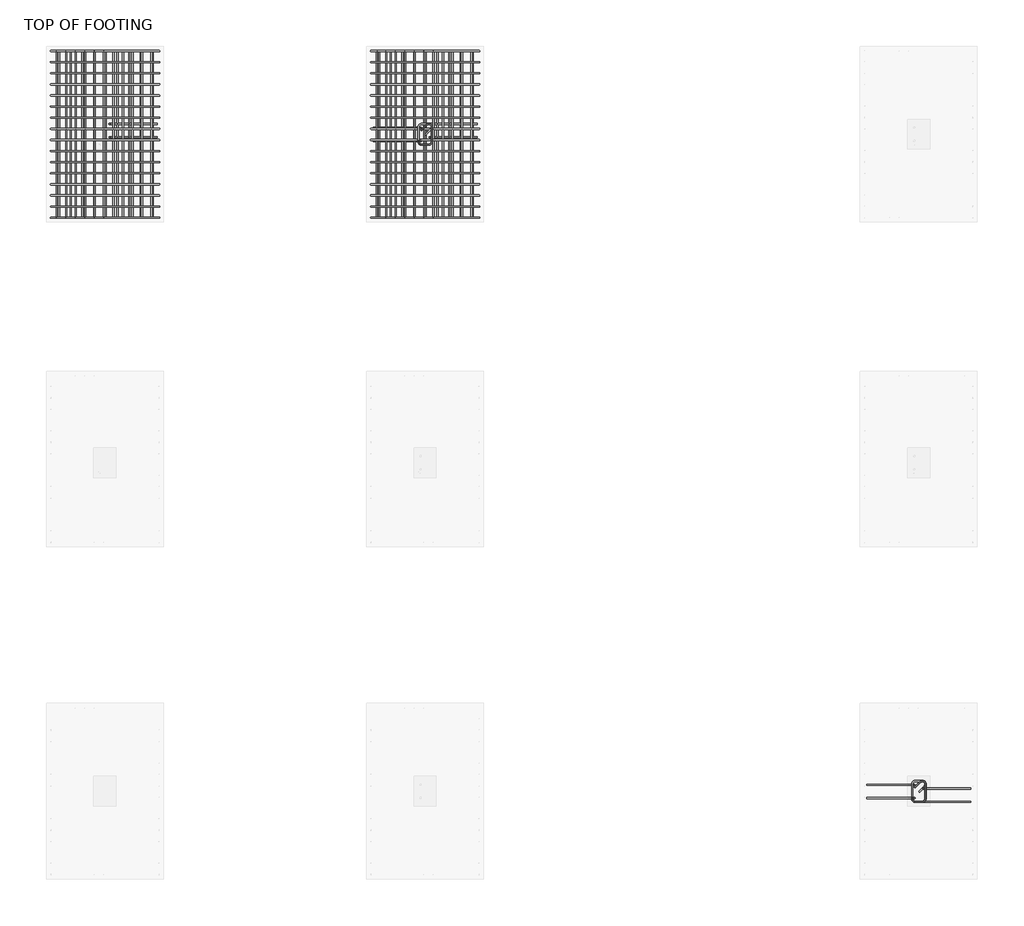
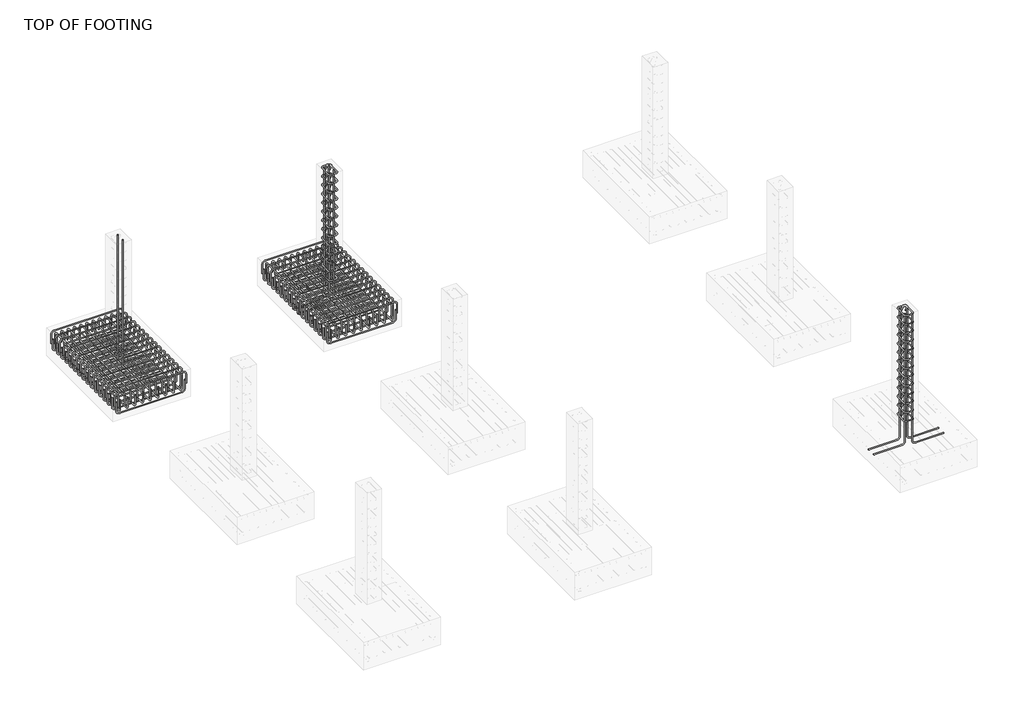
# One storey, part 4 of 8: 15 reinforcing bars.
"""IFC4 building model written with IfcOpenShell, lengths in millimetres."""

from ifc_helpers import new_model, si_unit, point, frame, origin, place, context, project, spatial, polyline, circle_curve, trimmed, segment, composite_curve, source, transform, mapped, element, save
from ifc_brep_helpers import swept_disk

model = new_model("IFC4")

# Units and contexts
model_context = context("Model", 3, world=origin())
ifc_project = project(units=[si_unit("LENGTHUNIT", "METRE", prefix="MILLI")], contexts=[model_context])

# Site, building, storey
site = spatial("IfcSite", under=ifc_project)
building = spatial("IfcBuilding", under=site)
storey = spatial("IfcBuildingStorey", under=building, Name="TOP OF FOOTING", Elevation=-1828.8)

# Reinforcing bars
placement = place(None, origin())
reinforcing_bar_shape = source(origin(), model_context, "Body", "SolidModel", [
    swept_disk(composite_curve([segment(polyline([(-4695.380398, 8895.4265586, -2177.1384798), (-5136.5372203, 8895.4265586, -2177.1384798)]), True, "CONTINUOUS"), segment(trimmed(circle_curve(frame((-5136.5372203, 8895.4265586, -2130.7884798), z_axis=(0.0, 1.0, 0.0), x_axis=(0.0, 0.0, -46.34999999999991)), 46.35), [point((-5136.5372203, 8895.4265586, -2177.1384798))], [point((-5182.8872203, 8895.4265586, -2130.7884798))], True, "CARTESIAN"), True, "CONTINUOUS"), segment(polyline([(-5182.8872203, 8895.4265586, -2130.7884798), (-5182.8872203, 8895.4265586, -40.0)]), True, "CONTINUOUS")], self_intersect=False), 6.35),
])
element("IfcReinforcingBar", 1, at=placement, inside=storey, context=model_context, shape_type="MappedRepresentation", body=[
    mapped(reinforcing_bar_shape, transform((0.0, 0.0, 0.0), x_axis=(1.0, 0.0, 0.0), y_axis=(0.0, 1.0, 0.0), z_axis=(0.0, 0.0, 1.0))),
    mapped(reinforcing_bar_shape, transform((0.0, 135.9, 0.0), x_axis=(1.0, 0.0, 0.0), y_axis=(0.0, 1.0, 0.0), z_axis=(0.0, 0.0, 1.0))),
])
reinforcing_bar_2_shape = source(origin(), model_context, "Body", "SolidModel", [
    swept_disk(composite_curve([segment(polyline([(-1993.1182423, 8966.4007933, -46.35), (-1937.3746793, 9022.1443562, -46.35)]), True, "CONTINUOUS"), segment(trimmed(circle_curve(frame((-1915.2068817, 8999.9765586, -46.35), z_axis=(0.0, 0.0, -1.0), x_axis=(-22.167797600000085, 22.167797600000995, 0.0)), 31.35), [point((-1937.3746793, 9022.1443562, -46.35))], [point((-1883.8568817, 8999.9765586, -46.35))], True, "CARTESIAN"), True, "CONTINUOUS"), segment(polyline([(-1883.8568817, 8999.9765586, -46.35), (-1883.8568817, 8850.5765586, -46.35)]), True, "CONTINUOUS"), segment(trimmed(circle_curve(frame((-1915.2068817, 8850.5765586, -46.35), z_axis=(0.0, 0.0, -1.0), x_axis=(31.34999999999991, 0.0, 0.0)), 31.35), [point((-1883.8568817, 8850.5765586, -46.35))], [point((-1915.2068817, 8819.2265586, -46.35))], True, "CARTESIAN"), True, "CONTINUOUS"), segment(polyline([(-1915.2068817, 8819.2265586, -46.35), (-1988.4068817, 8819.2265586, -46.35)]), True, "CONTINUOUS"), segment(trimmed(circle_curve(frame((-1988.4068817, 8850.5205096, -44.4761991), z_axis=(0.0, 0.05977036468717588, -0.9982121535551258), x_axis=(0.0, -31.29395100000147, -1.873800899999999)), 31.35), [point((-1988.4068817, 8819.2265586, -46.35))], [point((-2019.7568817, 8850.5205096, -44.4761991))], True, "CARTESIAN"), True, "CONTINUOUS"), segment(polyline([(-2019.7568817, 8850.5205096, -44.4761991), (-2019.7568817, 9000.0326076, -35.5238009)]), True, "CONTINUOUS"), segment(trimmed(circle_curve(frame((-1988.4068817, 9000.0326076, -35.5238009), z_axis=(0.0, 0.05977036468717588, -0.9982121535551258), x_axis=(-31.34999999999991, 0.0, 0.0)), 31.35), [point((-2019.7568817, 9000.0326076, -35.5238009))], [point((-1988.4068817, 9031.3265586, -33.65))], True, "CARTESIAN"), True, "CONTINUOUS"), segment(polyline([(-1988.4068817, 9031.3265586, -33.65), (-1915.2068817, 9031.3265586, -33.65)]), True, "CONTINUOUS"), segment(trimmed(circle_curve(frame((-1915.2068817, 8999.9765586, -33.65), z_axis=(0.0, 0.0, -1.0), x_axis=(0.0, 31.350000000000364, 0.0)), 31.35), [point((-1915.2068817, 9031.3265586, -33.65))], [point((-1893.0390841, 8977.808761, -33.65))], True, "CARTESIAN"), True, "CONTINUOUS"), segment(polyline([(-1893.0390841, 8977.808761, -33.65), (-1948.7826471, 8922.0651981, -33.65)]), True, "CONTINUOUS")], self_intersect=False), 6.35),
])
element("IfcReinforcingBar", 2, at=placement, inside=storey, context=model_context, shape_type="MappedRepresentation", body=[
    mapped(reinforcing_bar_2_shape, transform((0.0, 0.0, 0.0), x_axis=(1.0, 0.0, 0.0), y_axis=(0.0, 1.0, 0.0), z_axis=(0.0, 0.0, 1.0))),
    mapped(reinforcing_bar_2_shape, transform((0.0, 0.0, -144.675), x_axis=(1.0, 0.0, 0.0), y_axis=(0.0, 1.0, 0.0), z_axis=(0.0, 0.0, 1.0))),
    mapped(reinforcing_bar_2_shape, transform((0.0, 0.0, -289.35), x_axis=(1.0, 0.0, 0.0), y_axis=(0.0, 1.0, 0.0), z_axis=(0.0, 0.0, 1.0))),
    mapped(reinforcing_bar_2_shape, transform((0.0, 0.0, -434.025), x_axis=(1.0, 0.0, 0.0), y_axis=(0.0, 1.0, 0.0), z_axis=(0.0, 0.0, 1.0))),
    mapped(reinforcing_bar_2_shape, transform((0.0, 0.0, -578.7), x_axis=(1.0, 0.0, 0.0), y_axis=(0.0, 1.0, 0.0), z_axis=(0.0, 0.0, 1.0))),
    mapped(reinforcing_bar_2_shape, transform((0.0, 0.0, -723.375), x_axis=(1.0, 0.0, 0.0), y_axis=(0.0, 1.0, 0.0), z_axis=(0.0, 0.0, 1.0))),
    mapped(reinforcing_bar_2_shape, transform((0.0, 0.0, -868.05), x_axis=(1.0, 0.0, 0.0), y_axis=(0.0, 1.0, 0.0), z_axis=(0.0, 0.0, 1.0))),
    mapped(reinforcing_bar_2_shape, transform((0.0, 0.0, -1012.725), x_axis=(1.0, 0.0, 0.0), y_axis=(0.0, 1.0, 0.0), z_axis=(0.0, 0.0, 1.0))),
    mapped(reinforcing_bar_2_shape, transform((0.0, 0.0, -1157.4), x_axis=(1.0, 0.0, 0.0), y_axis=(0.0, 1.0, 0.0), z_axis=(0.0, 0.0, 1.0))),
    mapped(reinforcing_bar_2_shape, transform((0.0, 0.0, -1302.075), x_axis=(1.0, 0.0, 0.0), y_axis=(0.0, 1.0, 0.0), z_axis=(0.0, 0.0, 1.0))),
    mapped(reinforcing_bar_2_shape, transform((0.0, 0.0, -1446.75), x_axis=(1.0, 0.0, 0.0), y_axis=(0.0, 1.0, 0.0), z_axis=(0.0, 0.0, 1.0))),
    mapped(reinforcing_bar_2_shape, transform((0.0, 0.0, -1591.425), x_axis=(1.0, 0.0, 0.0), y_axis=(0.0, 1.0, 0.0), z_axis=(0.0, 0.0, 1.0))),
    mapped(reinforcing_bar_2_shape, transform((0.0, 0.0, -1736.1), x_axis=(1.0, 0.0, 0.0), y_axis=(0.0, 1.0, 0.0), z_axis=(0.0, 0.0, 1.0))),
])
reinforcing_bar_3_shape = source(origin(), model_context, "Body", "SolidModel", [
    swept_disk(composite_curve([segment(polyline([(-1418.780398, 8895.4265586, -2177.1384798), (-1859.9372203, 8895.4265586, -2177.1384798)]), True, "CONTINUOUS"), segment(trimmed(circle_curve(frame((-1859.9372203, 8895.4265586, -2130.7884798), z_axis=(0.0, 1.0, 0.0), x_axis=(0.0, 0.0, -46.34999999999991)), 46.35), [point((-1859.9372203, 8895.4265586, -2177.1384798))], [point((-1906.2872203, 8895.4265586, -2130.7884798))], True, "CARTESIAN"), True, "CONTINUOUS"), segment(polyline([(-1906.2872203, 8895.4265586, -2130.7884798), (-1906.2872203, 8895.4265586, -40.0)]), True, "CONTINUOUS")], self_intersect=False), 6.35),
])
element("IfcReinforcingBar", 3, at=placement, inside=storey, context=model_context, shape_type="MappedRepresentation", body=[
    mapped(reinforcing_bar_3_shape, transform((0.0, 0.0, 0.0), x_axis=(1.0, 0.0, 0.0), y_axis=(0.0, 1.0, 0.0), z_axis=(0.0, 0.0, 1.0))),
    mapped(reinforcing_bar_3_shape, transform((0.0, 135.9, 0.0), x_axis=(1.0, 0.0, 0.0), y_axis=(0.0, 1.0, 0.0), z_axis=(0.0, 0.0, 1.0))),
])
reinforcing_bar_4_shape = source(origin(), model_context, "Body", "SolidModel", [
    swept_disk(composite_curve([segment(polyline([(-2484.8333654, 8857.3265586, -2177.1384798), (-2043.6765432, 8857.3265586, -2177.1384798)]), True, "CONTINUOUS"), segment(trimmed(circle_curve(frame((-2043.6765432, 8857.3265586, -2130.7884798), z_axis=(0.0, -1.0, 0.0), x_axis=(0.0, 0.0, -46.34999999999991)), 46.35), [point((-2043.6765432, 8857.3265586, -2177.1384798))], [point((-1997.3265432, 8857.3265586, -2130.7884798))], True, "CARTESIAN"), True, "CONTINUOUS"), segment(polyline([(-1997.3265432, 8857.3265586, -2130.7884798), (-1997.3265432, 8857.3265586, -40.0)]), True, "CONTINUOUS")], self_intersect=False), 6.35),
])
element("IfcReinforcingBar", 4, at=placement, inside=storey, context=model_context, shape_type="MappedRepresentation", body=[
    mapped(reinforcing_bar_4_shape, transform((0.0, 0.0, 0.0), x_axis=(1.0, 0.0, 0.0), y_axis=(0.0, 1.0, 0.0), z_axis=(0.0, 0.0, 1.0))),
    mapped(reinforcing_bar_4_shape, transform((0.0, 135.9, 0.0), x_axis=(1.0, 0.0, 0.0), y_axis=(0.0, 1.0, 0.0), z_axis=(0.0, 0.0, 1.0))),
])
reinforcing_bar_5_shape = source(origin(), model_context, "Body", "SolidModel", [
    swept_disk(composite_curve([segment(polyline([(3061.4817577, 2235.4007933, -46.35), (3117.2253207, 2291.1443562, -46.35)]), True, "CONTINUOUS"), segment(trimmed(circle_curve(frame((3139.3931183, 2268.9765586, -46.35), z_axis=(0.0, 0.0, -1.0), x_axis=(-22.167797600000085, 22.167797600000085, 0.0)), 31.35), [point((3117.2253207, 2291.1443562, -46.35))], [point((3170.7431183, 2268.9765586, -46.35))], True, "CARTESIAN"), True, "CONTINUOUS"), segment(polyline([(3170.7431183, 2268.9765586, -46.35), (3170.7431183, 2119.5765586, -46.35)]), True, "CONTINUOUS"), segment(trimmed(circle_curve(frame((3139.3931183, 2119.5765586, -46.35), z_axis=(0.0, 0.0, -1.0), x_axis=(31.34999999999991, 0.0, 0.0)), 31.35), [point((3170.7431183, 2119.5765586, -46.35))], [point((3139.3931183, 2088.2265586, -46.35))], True, "CARTESIAN"), True, "CONTINUOUS"), segment(polyline([(3139.3931183, 2088.2265586, -46.35), (3066.1931183, 2088.2265586, -46.35)]), True, "CONTINUOUS"), segment(trimmed(circle_curve(frame((3066.1931183, 2119.5205096, -44.4761991), z_axis=(0.0, 0.05977036468717588, -0.9982121535551258), x_axis=(0.0, -31.293951000000106, -1.873800899999999)), 31.35), [point((3066.1931183, 2088.2265586, -46.35))], [point((3034.8431183, 2119.5205096, -44.4761991))], True, "CARTESIAN"), True, "CONTINUOUS"), segment(polyline([(3034.8431183, 2119.5205096, -44.4761991), (3034.8431183, 2269.0326076, -35.5238009)]), True, "CONTINUOUS"), segment(trimmed(circle_curve(frame((3066.1931183, 2269.0326076, -35.5238009), z_axis=(0.0, 0.05977036468717588, -0.9982121535551258), x_axis=(-31.350000000000364, 0.0, 0.0)), 31.35), [point((3034.8431183, 2269.0326076, -35.5238009))], [point((3066.1931183, 2300.3265586, -33.65))], True, "CARTESIAN"), True, "CONTINUOUS"), segment(polyline([(3066.1931183, 2300.3265586, -33.65), (3139.3931183, 2300.3265586, -33.65)]), True, "CONTINUOUS"), segment(trimmed(circle_curve(frame((3139.3931183, 2268.9765586, -33.65), z_axis=(0.0, 0.0, -1.0), x_axis=(0.0, 31.350000000000364, 0.0)), 31.35), [point((3139.3931183, 2300.3265586, -33.65))], [point((3161.5609159, 2246.808761, -33.65))], True, "CARTESIAN"), True, "CONTINUOUS"), segment(polyline([(3161.5609159, 2246.808761, -33.65), (3105.8173529, 2191.0651981, -33.65)]), True, "CONTINUOUS")], self_intersect=False), 6.35),
])
element("IfcReinforcingBar", 5, at=placement, inside=storey, context=model_context, shape_type="MappedRepresentation", body=[
    mapped(reinforcing_bar_5_shape, transform((0.0, 0.0, 0.0), x_axis=(1.0, 0.0, 0.0), y_axis=(0.0, 1.0, 0.0), z_axis=(0.0, 0.0, 1.0))),
    mapped(reinforcing_bar_5_shape, transform((0.0, 0.0, -144.675), x_axis=(1.0, 0.0, 0.0), y_axis=(0.0, 1.0, 0.0), z_axis=(0.0, 0.0, 1.0))),
    mapped(reinforcing_bar_5_shape, transform((0.0, 0.0, -289.35), x_axis=(1.0, 0.0, 0.0), y_axis=(0.0, 1.0, 0.0), z_axis=(0.0, 0.0, 1.0))),
    mapped(reinforcing_bar_5_shape, transform((0.0, 0.0, -434.025), x_axis=(1.0, 0.0, 0.0), y_axis=(0.0, 1.0, 0.0), z_axis=(0.0, 0.0, 1.0))),
    mapped(reinforcing_bar_5_shape, transform((0.0, 0.0, -578.7), x_axis=(1.0, 0.0, 0.0), y_axis=(0.0, 1.0, 0.0), z_axis=(0.0, 0.0, 1.0))),
    mapped(reinforcing_bar_5_shape, transform((0.0, 0.0, -723.375), x_axis=(1.0, 0.0, 0.0), y_axis=(0.0, 1.0, 0.0), z_axis=(0.0, 0.0, 1.0))),
    mapped(reinforcing_bar_5_shape, transform((0.0, 0.0, -868.05), x_axis=(1.0, 0.0, 0.0), y_axis=(0.0, 1.0, 0.0), z_axis=(0.0, 0.0, 1.0))),
    mapped(reinforcing_bar_5_shape, transform((0.0, 0.0, -1012.725), x_axis=(1.0, 0.0, 0.0), y_axis=(0.0, 1.0, 0.0), z_axis=(0.0, 0.0, 1.0))),
    mapped(reinforcing_bar_5_shape, transform((0.0, 0.0, -1157.4), x_axis=(1.0, 0.0, 0.0), y_axis=(0.0, 1.0, 0.0), z_axis=(0.0, 0.0, 1.0))),
    mapped(reinforcing_bar_5_shape, transform((0.0, 0.0, -1302.075), x_axis=(1.0, 0.0, 0.0), y_axis=(0.0, 1.0, 0.0), z_axis=(0.0, 0.0, 1.0))),
    mapped(reinforcing_bar_5_shape, transform((0.0, 0.0, -1446.75), x_axis=(1.0, 0.0, 0.0), y_axis=(0.0, 1.0, 0.0), z_axis=(0.0, 0.0, 1.0))),
    mapped(reinforcing_bar_5_shape, transform((0.0, 0.0, -1591.425), x_axis=(1.0, 0.0, 0.0), y_axis=(0.0, 1.0, 0.0), z_axis=(0.0, 0.0, 1.0))),
    mapped(reinforcing_bar_5_shape, transform((0.0, 0.0, -1736.1), x_axis=(1.0, 0.0, 0.0), y_axis=(0.0, 1.0, 0.0), z_axis=(0.0, 0.0, 1.0))),
])
reinforcing_bar_6_shape = source(origin(), model_context, "Body", "SolidModel", [
    swept_disk(composite_curve([segment(polyline([(3635.819602, 2088.2265586, -2177.1384798), (3194.6627797, 2088.2265586, -2177.1384798)]), True, "CONTINUOUS"), segment(trimmed(circle_curve(frame((3194.6627797, 2088.2265586, -2130.7884798), z_axis=(0.0, 1.0, 0.0), x_axis=(0.0, 0.0, -46.34999999999991)), 46.35), [point((3194.6627797, 2088.2265586, -2177.1384798))], [point((3148.3127797, 2088.2265586, -2130.7884798))], True, "CARTESIAN"), True, "CONTINUOUS"), segment(polyline([(3148.3127797, 2088.2265586, -2130.7884798), (3148.3127797, 2088.2265586, -40.0)]), True, "CONTINUOUS")], self_intersect=False), 6.35),
])
element("IfcReinforcingBar", 6, at=placement, inside=storey, context=model_context, shape_type="MappedRepresentation", body=[
    mapped(reinforcing_bar_6_shape, transform((0.0, 0.0, 0.0), x_axis=(1.0, 0.0, 0.0), y_axis=(0.0, 1.0, 0.0), z_axis=(0.0, 0.0, 1.0))),
    mapped(reinforcing_bar_6_shape, transform((0.0, 135.9, 0.0), x_axis=(1.0, 0.0, 0.0), y_axis=(0.0, 1.0, 0.0), z_axis=(0.0, 0.0, 1.0))),
])
reinforcing_bar_7_shape = source(origin(), model_context, "Body", "SolidModel", [
    swept_disk(composite_curve([segment(polyline([(2569.7666346, 2126.3265586, -2177.1384798), (3010.9234568, 2126.3265586, -2177.1384798)]), True, "CONTINUOUS"), segment(trimmed(circle_curve(frame((3010.9234568, 2126.3265586, -2130.7884798), z_axis=(0.0, -1.0, 0.0), x_axis=(0.0, 0.0, -46.34999999999991)), 46.35), [point((3010.9234568, 2126.3265586, -2177.1384798))], [point((3057.2734568, 2126.3265586, -2130.7884798))], True, "CARTESIAN"), True, "CONTINUOUS"), segment(polyline([(3057.2734568, 2126.3265586, -2130.7884798), (3057.2734568, 2126.3265586, -40.0)]), True, "CONTINUOUS")], self_intersect=False), 6.35),
])
element("IfcReinforcingBar", 7, at=placement, inside=storey, context=model_context, shape_type="MappedRepresentation", body=[
    mapped(reinforcing_bar_7_shape, transform((0.0, 0.0, 0.0), x_axis=(1.0, 0.0, 0.0), y_axis=(0.0, 1.0, 0.0), z_axis=(0.0, 0.0, 1.0))),
    mapped(reinforcing_bar_7_shape, transform((0.0, 135.9, 0.0), x_axis=(1.0, 0.0, 0.0), y_axis=(0.0, 1.0, 0.0), z_axis=(0.0, 0.0, 1.0))),
])
reinforcing_bar_8_shape = source(origin(), model_context, "Body", "SolidModel", [
    swept_disk(composite_curve([segment(polyline([(-4694.1573229, 9778.9265586, -2008.2544267), (-4694.1573229, 9778.9265586, -2155.5544267)]), True, "CONTINUOUS"), segment(trimmed(circle_curve(frame((-4740.5073229, 9778.9265586, -2155.5544267), z_axis=(0.0, 1.0, 0.0), x_axis=(46.350000000000364, 0.0, 0.0)), 46.35), [point((-4694.1573229, 9778.9265586, -2155.5544267))], [point((-4740.5073229, 9778.9265586, -2201.9044267))], True, "CARTESIAN"), True, "CONTINUOUS"), segment(polyline([(-4740.5073229, 9778.9265586, -2201.9044267), (-5711.5233592, 9778.9265586, -2201.9044267)]), True, "CONTINUOUS"), segment(trimmed(circle_curve(frame((-5711.5233592, 9778.9265586, -2155.5544267), z_axis=(0.0, 1.0, 0.0), x_axis=(0.0, 0.0, -46.34999999999991)), 46.35), [point((-5711.5233592, 9778.9265586, -2201.9044267))], [point((-5757.8733592, 9778.9265586, -2155.5544267))], True, "CARTESIAN"), True, "CONTINUOUS"), segment(polyline([(-5757.8733592, 9778.9265586, -2155.5544267), (-5757.8733592, 9778.9265586, -2008.2544267)]), True, "CONTINUOUS")], self_intersect=False), 6.35),
])
element("IfcReinforcingBar", 8, at=placement, inside=storey, context=model_context, shape_type="MappedRepresentation", body=[
    mapped(reinforcing_bar_8_shape, transform((0.0, 0.0, 0.0), x_axis=(1.0, 0.0, 0.0), y_axis=(0.0, 1.0, 0.0), z_axis=(0.0, 0.0, 1.0))),
    mapped(reinforcing_bar_8_shape, transform((0.0, -113.82, 0.0), x_axis=(1.0, 0.0, 0.0), y_axis=(0.0, 1.0, 0.0), z_axis=(0.0, 0.0, 1.0))),
    mapped(reinforcing_bar_8_shape, transform((0.0, -227.64, 0.0), x_axis=(1.0, 0.0, 0.0), y_axis=(0.0, 1.0, 0.0), z_axis=(0.0, 0.0, 1.0))),
    mapped(reinforcing_bar_8_shape, transform((0.0, -341.46, 0.0), x_axis=(1.0, 0.0, 0.0), y_axis=(0.0, 1.0, 0.0), z_axis=(0.0, 0.0, 1.0))),
    mapped(reinforcing_bar_8_shape, transform((0.0, -455.28, 0.0), x_axis=(1.0, 0.0, 0.0), y_axis=(0.0, 1.0, 0.0), z_axis=(0.0, 0.0, 1.0))),
    mapped(reinforcing_bar_8_shape, transform((0.0, -569.1, 0.0), x_axis=(1.0, 0.0, 0.0), y_axis=(0.0, 1.0, 0.0), z_axis=(0.0, 0.0, 1.0))),
    mapped(reinforcing_bar_8_shape, transform((0.0, -682.92, 0.0), x_axis=(1.0, 0.0, 0.0), y_axis=(0.0, 1.0, 0.0), z_axis=(0.0, 0.0, 1.0))),
    mapped(reinforcing_bar_8_shape, transform((0.0, -796.74, 0.0), x_axis=(1.0, 0.0, 0.0), y_axis=(0.0, 1.0, 0.0), z_axis=(0.0, 0.0, 1.0))),
    mapped(reinforcing_bar_8_shape, transform((0.0, -910.56, 0.0), x_axis=(1.0, 0.0, 0.0), y_axis=(0.0, 1.0, 0.0), z_axis=(0.0, 0.0, 1.0))),
    mapped(reinforcing_bar_8_shape, transform((0.0, -1024.38, 0.0), x_axis=(1.0, 0.0, 0.0), y_axis=(0.0, 1.0, 0.0), z_axis=(0.0, 0.0, 1.0))),
    mapped(reinforcing_bar_8_shape, transform((0.0, -1138.2, 0.0), x_axis=(1.0, 0.0, 0.0), y_axis=(0.0, 1.0, 0.0), z_axis=(0.0, 0.0, 1.0))),
    mapped(reinforcing_bar_8_shape, transform((0.0, -1252.02, 0.0), x_axis=(1.0, 0.0, 0.0), y_axis=(0.0, 1.0, 0.0), z_axis=(0.0, 0.0, 1.0))),
    mapped(reinforcing_bar_8_shape, transform((0.0, -1365.84, 0.0), x_axis=(1.0, 0.0, 0.0), y_axis=(0.0, 1.0, 0.0), z_axis=(0.0, 0.0, 1.0))),
    mapped(reinforcing_bar_8_shape, transform((0.0, -1479.66, 0.0), x_axis=(1.0, 0.0, 0.0), y_axis=(0.0, 1.0, 0.0), z_axis=(0.0, 0.0, 1.0))),
    mapped(reinforcing_bar_8_shape, transform((0.0, -1593.48, 0.0), x_axis=(1.0, 0.0, 0.0), y_axis=(0.0, 1.0, 0.0), z_axis=(0.0, 0.0, 1.0))),
    mapped(reinforcing_bar_8_shape, transform((0.0, -1707.3, 0.0), x_axis=(1.0, 0.0, 0.0), y_axis=(0.0, 1.0, 0.0), z_axis=(0.0, 0.0, 1.0))),
])
reinforcing_bar_9_shape = source(origin(), model_context, "Body", "SolidModel", [
    swept_disk(composite_curve([segment(polyline([(-5782.0568817, 9778.9265586, -2068.8), (-5782.0568817, 9778.9265586, -1921.5)]), True, "CONTINUOUS"), segment(trimmed(circle_curve(frame((-5735.7068817, 9778.9265586, -1921.5), z_axis=(0.0, 1.0, 0.0), x_axis=(-46.350000000000364, 0.0, 0.0)), 46.35), [point((-5782.0568817, 9778.9265586, -1921.5))], [point((-5735.7068817, 9778.9265586, -1875.15))], True, "CARTESIAN"), True, "CONTINUOUS"), segment(polyline([(-5735.7068817, 9778.9265586, -1875.15), (-4721.1068817, 9778.9265586, -1875.15)]), True, "CONTINUOUS"), segment(trimmed(circle_curve(frame((-4721.1068817, 9778.9265586, -1921.5), z_axis=(0.0, 1.0, 0.0), x_axis=(0.0, 0.0, 46.34999999999991)), 46.35), [point((-4721.1068817, 9778.9265586, -1875.15))], [point((-4674.7568817, 9778.9265586, -1921.5))], True, "CARTESIAN"), True, "CONTINUOUS"), segment(polyline([(-4674.7568817, 9778.9265586, -1921.5), (-4674.7568817, 9778.9265586, -2068.8)]), True, "CONTINUOUS")], self_intersect=False), 6.35),
])
element("IfcReinforcingBar", 9, at=placement, inside=storey, context=model_context, shape_type="MappedRepresentation", body=[
    mapped(reinforcing_bar_9_shape, transform((0.0, 0.0, 0.0), x_axis=(1.0, 0.0, 0.0), y_axis=(0.0, 1.0, 0.0), z_axis=(0.0, 0.0, 1.0))),
    mapped(reinforcing_bar_9_shape, transform((0.0, -113.82, 0.0), x_axis=(1.0, 0.0, 0.0), y_axis=(0.0, 1.0, 0.0), z_axis=(0.0, 0.0, 1.0))),
    mapped(reinforcing_bar_9_shape, transform((0.0, -227.64, 0.0), x_axis=(1.0, 0.0, 0.0), y_axis=(0.0, 1.0, 0.0), z_axis=(0.0, 0.0, 1.0))),
    mapped(reinforcing_bar_9_shape, transform((0.0, -341.46, 0.0), x_axis=(1.0, 0.0, 0.0), y_axis=(0.0, 1.0, 0.0), z_axis=(0.0, 0.0, 1.0))),
    mapped(reinforcing_bar_9_shape, transform((0.0, -455.28, 0.0), x_axis=(1.0, 0.0, 0.0), y_axis=(0.0, 1.0, 0.0), z_axis=(0.0, 0.0, 1.0))),
    mapped(reinforcing_bar_9_shape, transform((0.0, -569.1, 0.0), x_axis=(1.0, 0.0, 0.0), y_axis=(0.0, 1.0, 0.0), z_axis=(0.0, 0.0, 1.0))),
    mapped(reinforcing_bar_9_shape, transform((0.0, -682.92, 0.0), x_axis=(1.0, 0.0, 0.0), y_axis=(0.0, 1.0, 0.0), z_axis=(0.0, 0.0, 1.0))),
    mapped(reinforcing_bar_9_shape, transform((0.0, -796.74, 0.0), x_axis=(1.0, 0.0, 0.0), y_axis=(0.0, 1.0, 0.0), z_axis=(0.0, 0.0, 1.0))),
    mapped(reinforcing_bar_9_shape, transform((0.0, -910.56, 0.0), x_axis=(1.0, 0.0, 0.0), y_axis=(0.0, 1.0, 0.0), z_axis=(0.0, 0.0, 1.0))),
    mapped(reinforcing_bar_9_shape, transform((0.0, -1024.38, 0.0), x_axis=(1.0, 0.0, 0.0), y_axis=(0.0, 1.0, 0.0), z_axis=(0.0, 0.0, 1.0))),
    mapped(reinforcing_bar_9_shape, transform((0.0, -1138.2, 0.0), x_axis=(1.0, 0.0, 0.0), y_axis=(0.0, 1.0, 0.0), z_axis=(0.0, 0.0, 1.0))),
    mapped(reinforcing_bar_9_shape, transform((0.0, -1252.02, 0.0), x_axis=(1.0, 0.0, 0.0), y_axis=(0.0, 1.0, 0.0), z_axis=(0.0, 0.0, 1.0))),
    mapped(reinforcing_bar_9_shape, transform((0.0, -1365.84, 0.0), x_axis=(1.0, 0.0, 0.0), y_axis=(0.0, 1.0, 0.0), z_axis=(0.0, 0.0, 1.0))),
    mapped(reinforcing_bar_9_shape, transform((0.0, -1479.66, 0.0), x_axis=(1.0, 0.0, 0.0), y_axis=(0.0, 1.0, 0.0), z_axis=(0.0, 0.0, 1.0))),
    mapped(reinforcing_bar_9_shape, transform((0.0, -1593.48, 0.0), x_axis=(1.0, 0.0, 0.0), y_axis=(0.0, 1.0, 0.0), z_axis=(0.0, 0.0, 1.0))),
    mapped(reinforcing_bar_9_shape, transform((0.0, -1707.3, 0.0), x_axis=(1.0, 0.0, 0.0), y_axis=(0.0, 1.0, 0.0), z_axis=(0.0, 0.0, 1.0))),
])
reinforcing_bar_10_shape = source(origin(), model_context, "Body", "SolidModel", [
    swept_disk(composite_curve([segment(polyline([(-5699.8348303, 9778.9265586, -1986.9111268), (-5699.8348303, 9778.9265586, -2134.2111268)]), True, "CONTINUOUS"), segment(trimmed(circle_curve(frame((-5699.8348303, 9732.5765586, -2134.2111268), z_axis=(-1.0, 0.0, 0.0), x_axis=(0.0, 46.350000000000364, 0.0)), 46.35), [point((-5699.8348303, 9778.9265586, -2134.2111268))], [point((-5699.8348303, 9732.5765586, -2180.5611268))], True, "CARTESIAN"), True, "CONTINUOUS"), segment(polyline([(-5699.8348303, 9732.5765586, -2180.5611268), (-5699.8348303, 8117.9765586, -2180.5611268)]), True, "CONTINUOUS"), segment(trimmed(circle_curve(frame((-5699.8348303, 8117.9765586, -2134.2111268), z_axis=(-1.0, 0.0, 0.0), x_axis=(0.0, 0.0, -46.34999999999991)), 46.35), [point((-5699.8348303, 8117.9765586, -2180.5611268))], [point((-5699.8348303, 8071.6265586, -2134.2111268))], True, "CARTESIAN"), True, "CONTINUOUS"), segment(polyline([(-5699.8348303, 8071.6265586, -2134.2111268), (-5699.8348303, 8071.6265586, -1986.9111268)]), True, "CONTINUOUS")], self_intersect=False), 6.35),
])
element("IfcReinforcingBar", 10, at=placement, inside=storey, context=model_context, shape_type="MappedRepresentation", body=[
    mapped(reinforcing_bar_10_shape, transform((0.0, 0.0, 0.0), x_axis=(1.0, 0.0, 0.0), y_axis=(0.0, 1.0, 0.0), z_axis=(0.0, 0.0, 1.0))),
    mapped(reinforcing_bar_10_shape, transform((119.5564677, 0.0, 0.0), x_axis=(1.0, 0.0, 0.0), y_axis=(0.0, 1.0, 0.0), z_axis=(0.0, 0.0, 1.0))),
    mapped(reinforcing_bar_10_shape, transform((239.1129355, 0.0, 0.0), x_axis=(1.0, 0.0, 0.0), y_axis=(0.0, 1.0, 0.0), z_axis=(0.0, 0.0, 1.0))),
    mapped(reinforcing_bar_10_shape, transform((358.6694032, 0.0, 0.0), x_axis=(1.0, 0.0, 0.0), y_axis=(0.0, 1.0, 0.0), z_axis=(0.0, 0.0, 1.0))),
    mapped(reinforcing_bar_10_shape, transform((478.2258709, 0.0, 0.0), x_axis=(1.0, 0.0, 0.0), y_axis=(0.0, 1.0, 0.0), z_axis=(0.0, 0.0, 1.0))),
    mapped(reinforcing_bar_10_shape, transform((597.7823387, 0.0, 0.0), x_axis=(1.0, 0.0, 0.0), y_axis=(0.0, 1.0, 0.0), z_axis=(0.0, 0.0, 1.0))),
    mapped(reinforcing_bar_10_shape, transform((717.3388064, 0.0, 0.0), x_axis=(1.0, 0.0, 0.0), y_axis=(0.0, 1.0, 0.0), z_axis=(0.0, 0.0, 1.0))),
    mapped(reinforcing_bar_10_shape, transform((836.8952741, 0.0, 0.0), x_axis=(1.0, 0.0, 0.0), y_axis=(0.0, 1.0, 0.0), z_axis=(0.0, 0.0, 1.0))),
    mapped(reinforcing_bar_10_shape, transform((956.4517419, 0.0, 0.0), x_axis=(1.0, 0.0, 0.0), y_axis=(0.0, 1.0, 0.0), z_axis=(0.0, 0.0, 1.0))),
])
reinforcing_bar_11_shape = source(origin(), model_context, "Body", "SolidModel", [
    swept_disk(composite_curve([segment(polyline([(-4754.0668299, 9778.9265586, -2094.8977257), (-4754.0668299, 9778.9265586, -1947.5977257)]), True, "CONTINUOUS"), segment(trimmed(circle_curve(frame((-4754.0668299, 9732.5765586, -1947.5977257), z_axis=(1.0, 0.0, 0.0), x_axis=(0.0, 46.350000000000364, 0.0)), 46.35), [point((-4754.0668299, 9778.9265586, -1947.5977257))], [point((-4754.0668299, 9732.5765586, -1901.2477257))], True, "CARTESIAN"), True, "CONTINUOUS"), segment(polyline([(-4754.0668299, 9732.5765586, -1901.2477257), (-4754.0668299, 8117.9765586, -1901.2477257)]), True, "CONTINUOUS"), segment(trimmed(circle_curve(frame((-4754.0668299, 8117.9765586, -1947.5977257), z_axis=(1.0, 0.0, 0.0), x_axis=(0.0, 0.0, 46.34999999999991)), 46.35), [point((-4754.0668299, 8117.9765586, -1901.2477257))], [point((-4754.0668299, 8071.6265586, -1947.5977257))], True, "CARTESIAN"), True, "CONTINUOUS"), segment(polyline([(-4754.0668299, 8071.6265586, -1947.5977257), (-4754.0668299, 8071.6265586, -2094.8977257)]), True, "CONTINUOUS")], self_intersect=False), 6.35),
])
element("IfcReinforcingBar", 11, at=placement, inside=storey, context=model_context, shape_type="MappedRepresentation", body=[
    mapped(reinforcing_bar_11_shape, transform((0.0, 0.0, 0.0), x_axis=(1.0, 0.0, 0.0), y_axis=(0.0, 1.0, 0.0), z_axis=(0.0, 0.0, 1.0))),
    mapped(reinforcing_bar_11_shape, transform((-97.0050815, 0.0, 0.0), x_axis=(1.0, 0.0, 0.0), y_axis=(0.0, 1.0, 0.0), z_axis=(0.0, 0.0, 1.0))),
    mapped(reinforcing_bar_11_shape, transform((-194.0101631, 0.0, 0.0), x_axis=(1.0, 0.0, 0.0), y_axis=(0.0, 1.0, 0.0), z_axis=(0.0, 0.0, 1.0))),
    mapped(reinforcing_bar_11_shape, transform((-291.0152446, 0.0, 0.0), x_axis=(1.0, 0.0, 0.0), y_axis=(0.0, 1.0, 0.0), z_axis=(0.0, 0.0, 1.0))),
    mapped(reinforcing_bar_11_shape, transform((-388.0203261, 0.0, 0.0), x_axis=(1.0, 0.0, 0.0), y_axis=(0.0, 1.0, 0.0), z_axis=(0.0, 0.0, 1.0))),
    mapped(reinforcing_bar_11_shape, transform((-485.0254076, 0.0, 0.0), x_axis=(1.0, 0.0, 0.0), y_axis=(0.0, 1.0, 0.0), z_axis=(0.0, 0.0, 1.0))),
    mapped(reinforcing_bar_11_shape, transform((-582.0304892, 0.0, 0.0), x_axis=(1.0, 0.0, 0.0), y_axis=(0.0, 1.0, 0.0), z_axis=(0.0, 0.0, 1.0))),
    mapped(reinforcing_bar_11_shape, transform((-679.0355707, 0.0, 0.0), x_axis=(1.0, 0.0, 0.0), y_axis=(0.0, 1.0, 0.0), z_axis=(0.0, 0.0, 1.0))),
    mapped(reinforcing_bar_11_shape, transform((-776.0406522, 0.0, 0.0), x_axis=(1.0, 0.0, 0.0), y_axis=(0.0, 1.0, 0.0), z_axis=(0.0, 0.0, 1.0))),
    mapped(reinforcing_bar_11_shape, transform((-873.0457338, 0.0, 0.0), x_axis=(1.0, 0.0, 0.0), y_axis=(0.0, 1.0, 0.0), z_axis=(0.0, 0.0, 1.0))),
    mapped(reinforcing_bar_11_shape, transform((-970.0508153, 0.0, 0.0), x_axis=(1.0, 0.0, 0.0), y_axis=(0.0, 1.0, 0.0), z_axis=(0.0, 0.0, 1.0))),
])
reinforcing_bar_12_shape = source(origin(), model_context, "Body", "SolidModel", [
    swept_disk(composite_curve([segment(polyline([(-1417.5573229, 9778.9265586, -2008.2544267), (-1417.5573229, 9778.9265586, -2155.5544267)]), True, "CONTINUOUS"), segment(trimmed(circle_curve(frame((-1463.9073229, 9778.9265586, -2155.5544267), z_axis=(0.0, 1.0, 0.0), x_axis=(46.350000000000136, 0.0, 0.0)), 46.35), [point((-1417.5573229, 9778.9265586, -2155.5544267))], [point((-1463.9073229, 9778.9265586, -2201.9044267))], True, "CARTESIAN"), True, "CONTINUOUS"), segment(polyline([(-1463.9073229, 9778.9265586, -2201.9044267), (-2434.9233592, 9778.9265586, -2201.9044267)]), True, "CONTINUOUS"), segment(trimmed(circle_curve(frame((-2434.9233592, 9778.9265586, -2155.5544267), z_axis=(0.0, 1.0, 0.0), x_axis=(0.0, 0.0, -46.34999999999991)), 46.35), [point((-2434.9233592, 9778.9265586, -2201.9044267))], [point((-2481.2733592, 9778.9265586, -2155.5544267))], True, "CARTESIAN"), True, "CONTINUOUS"), segment(polyline([(-2481.2733592, 9778.9265586, -2155.5544267), (-2481.2733592, 9778.9265586, -2008.2544267)]), True, "CONTINUOUS")], self_intersect=False), 6.35),
])
element("IfcReinforcingBar", 12, at=placement, inside=storey, context=model_context, shape_type="MappedRepresentation", body=[
    mapped(reinforcing_bar_12_shape, transform((0.0, 0.0, 0.0), x_axis=(1.0, 0.0, 0.0), y_axis=(0.0, 1.0, 0.0), z_axis=(0.0, 0.0, 1.0))),
    mapped(reinforcing_bar_12_shape, transform((0.0, -113.82, 0.0), x_axis=(1.0, 0.0, 0.0), y_axis=(0.0, 1.0, 0.0), z_axis=(0.0, 0.0, 1.0))),
    mapped(reinforcing_bar_12_shape, transform((0.0, -227.64, 0.0), x_axis=(1.0, 0.0, 0.0), y_axis=(0.0, 1.0, 0.0), z_axis=(0.0, 0.0, 1.0))),
    mapped(reinforcing_bar_12_shape, transform((0.0, -341.46, 0.0), x_axis=(1.0, 0.0, 0.0), y_axis=(0.0, 1.0, 0.0), z_axis=(0.0, 0.0, 1.0))),
    mapped(reinforcing_bar_12_shape, transform((0.0, -455.28, 0.0), x_axis=(1.0, 0.0, 0.0), y_axis=(0.0, 1.0, 0.0), z_axis=(0.0, 0.0, 1.0))),
    mapped(reinforcing_bar_12_shape, transform((0.0, -569.1, 0.0), x_axis=(1.0, 0.0, 0.0), y_axis=(0.0, 1.0, 0.0), z_axis=(0.0, 0.0, 1.0))),
    mapped(reinforcing_bar_12_shape, transform((0.0, -682.92, 0.0), x_axis=(1.0, 0.0, 0.0), y_axis=(0.0, 1.0, 0.0), z_axis=(0.0, 0.0, 1.0))),
    mapped(reinforcing_bar_12_shape, transform((0.0, -796.74, 0.0), x_axis=(1.0, 0.0, 0.0), y_axis=(0.0, 1.0, 0.0), z_axis=(0.0, 0.0, 1.0))),
    mapped(reinforcing_bar_12_shape, transform((0.0, -910.56, 0.0), x_axis=(1.0, 0.0, 0.0), y_axis=(0.0, 1.0, 0.0), z_axis=(0.0, 0.0, 1.0))),
    mapped(reinforcing_bar_12_shape, transform((0.0, -1024.38, 0.0), x_axis=(1.0, 0.0, 0.0), y_axis=(0.0, 1.0, 0.0), z_axis=(0.0, 0.0, 1.0))),
    mapped(reinforcing_bar_12_shape, transform((0.0, -1138.2, 0.0), x_axis=(1.0, 0.0, 0.0), y_axis=(0.0, 1.0, 0.0), z_axis=(0.0, 0.0, 1.0))),
    mapped(reinforcing_bar_12_shape, transform((0.0, -1252.02, 0.0), x_axis=(1.0, 0.0, 0.0), y_axis=(0.0, 1.0, 0.0), z_axis=(0.0, 0.0, 1.0))),
    mapped(reinforcing_bar_12_shape, transform((0.0, -1365.84, 0.0), x_axis=(1.0, 0.0, 0.0), y_axis=(0.0, 1.0, 0.0), z_axis=(0.0, 0.0, 1.0))),
    mapped(reinforcing_bar_12_shape, transform((0.0, -1479.66, 0.0), x_axis=(1.0, 0.0, 0.0), y_axis=(0.0, 1.0, 0.0), z_axis=(0.0, 0.0, 1.0))),
    mapped(reinforcing_bar_12_shape, transform((0.0, -1593.48, 0.0), x_axis=(1.0, 0.0, 0.0), y_axis=(0.0, 1.0, 0.0), z_axis=(0.0, 0.0, 1.0))),
    mapped(reinforcing_bar_12_shape, transform((0.0, -1707.3, 0.0), x_axis=(1.0, 0.0, 0.0), y_axis=(0.0, 1.0, 0.0), z_axis=(0.0, 0.0, 1.0))),
])
reinforcing_bar_13_shape = source(origin(), model_context, "Body", "SolidModel", [
    swept_disk(composite_curve([segment(polyline([(-2505.4568817, 9778.9265586, -2068.8), (-2505.4568817, 9778.9265586, -1921.5)]), True, "CONTINUOUS"), segment(trimmed(circle_curve(frame((-2459.1068817, 9778.9265586, -1921.5), z_axis=(0.0, 1.0, 0.0), x_axis=(-46.34999999999991, 0.0, 0.0)), 46.35), [point((-2505.4568817, 9778.9265586, -1921.5))], [point((-2459.1068817, 9778.9265586, -1875.15))], True, "CARTESIAN"), True, "CONTINUOUS"), segment(polyline([(-2459.1068817, 9778.9265586, -1875.15), (-1444.5068817, 9778.9265586, -1875.15)]), True, "CONTINUOUS"), segment(trimmed(circle_curve(frame((-1444.5068817, 9778.9265586, -1921.5), z_axis=(0.0, 1.0, 0.0), x_axis=(0.0, 0.0, 46.34999999999991)), 46.35), [point((-1444.5068817, 9778.9265586, -1875.15))], [point((-1398.1568817, 9778.9265586, -1921.5))], True, "CARTESIAN"), True, "CONTINUOUS"), segment(polyline([(-1398.1568817, 9778.9265586, -1921.5), (-1398.1568817, 9778.9265586, -2068.8)]), True, "CONTINUOUS")], self_intersect=False), 6.35),
])
element("IfcReinforcingBar", 13, at=placement, inside=storey, context=model_context, shape_type="MappedRepresentation", body=[
    mapped(reinforcing_bar_13_shape, transform((0.0, 0.0, 0.0), x_axis=(1.0, 0.0, 0.0), y_axis=(0.0, 1.0, 0.0), z_axis=(0.0, 0.0, 1.0))),
    mapped(reinforcing_bar_13_shape, transform((0.0, -113.82, 0.0), x_axis=(1.0, 0.0, 0.0), y_axis=(0.0, 1.0, 0.0), z_axis=(0.0, 0.0, 1.0))),
    mapped(reinforcing_bar_13_shape, transform((0.0, -227.64, 0.0), x_axis=(1.0, 0.0, 0.0), y_axis=(0.0, 1.0, 0.0), z_axis=(0.0, 0.0, 1.0))),
    mapped(reinforcing_bar_13_shape, transform((0.0, -341.46, 0.0), x_axis=(1.0, 0.0, 0.0), y_axis=(0.0, 1.0, 0.0), z_axis=(0.0, 0.0, 1.0))),
    mapped(reinforcing_bar_13_shape, transform((0.0, -455.28, 0.0), x_axis=(1.0, 0.0, 0.0), y_axis=(0.0, 1.0, 0.0), z_axis=(0.0, 0.0, 1.0))),
    mapped(reinforcing_bar_13_shape, transform((0.0, -569.1, 0.0), x_axis=(1.0, 0.0, 0.0), y_axis=(0.0, 1.0, 0.0), z_axis=(0.0, 0.0, 1.0))),
    mapped(reinforcing_bar_13_shape, transform((0.0, -682.92, 0.0), x_axis=(1.0, 0.0, 0.0), y_axis=(0.0, 1.0, 0.0), z_axis=(0.0, 0.0, 1.0))),
    mapped(reinforcing_bar_13_shape, transform((0.0, -796.74, 0.0), x_axis=(1.0, 0.0, 0.0), y_axis=(0.0, 1.0, 0.0), z_axis=(0.0, 0.0, 1.0))),
    mapped(reinforcing_bar_13_shape, transform((0.0, -910.56, 0.0), x_axis=(1.0, 0.0, 0.0), y_axis=(0.0, 1.0, 0.0), z_axis=(0.0, 0.0, 1.0))),
    mapped(reinforcing_bar_13_shape, transform((0.0, -1024.38, 0.0), x_axis=(1.0, 0.0, 0.0), y_axis=(0.0, 1.0, 0.0), z_axis=(0.0, 0.0, 1.0))),
    mapped(reinforcing_bar_13_shape, transform((0.0, -1138.2, 0.0), x_axis=(1.0, 0.0, 0.0), y_axis=(0.0, 1.0, 0.0), z_axis=(0.0, 0.0, 1.0))),
    mapped(reinforcing_bar_13_shape, transform((0.0, -1252.02, 0.0), x_axis=(1.0, 0.0, 0.0), y_axis=(0.0, 1.0, 0.0), z_axis=(0.0, 0.0, 1.0))),
    mapped(reinforcing_bar_13_shape, transform((0.0, -1365.84, 0.0), x_axis=(1.0, 0.0, 0.0), y_axis=(0.0, 1.0, 0.0), z_axis=(0.0, 0.0, 1.0))),
    mapped(reinforcing_bar_13_shape, transform((0.0, -1479.66, 0.0), x_axis=(1.0, 0.0, 0.0), y_axis=(0.0, 1.0, 0.0), z_axis=(0.0, 0.0, 1.0))),
    mapped(reinforcing_bar_13_shape, transform((0.0, -1593.48, 0.0), x_axis=(1.0, 0.0, 0.0), y_axis=(0.0, 1.0, 0.0), z_axis=(0.0, 0.0, 1.0))),
    mapped(reinforcing_bar_13_shape, transform((0.0, -1707.3, 0.0), x_axis=(1.0, 0.0, 0.0), y_axis=(0.0, 1.0, 0.0), z_axis=(0.0, 0.0, 1.0))),
])
reinforcing_bar_14_shape = source(origin(), model_context, "Body", "SolidModel", [
    swept_disk(composite_curve([segment(polyline([(-2423.2348303, 9778.9265586, -1986.9111268), (-2423.2348303, 9778.9265586, -2134.2111268)]), True, "CONTINUOUS"), segment(trimmed(circle_curve(frame((-2423.2348303, 9732.5765586, -2134.2111268), z_axis=(-1.0, 0.0, 0.0), x_axis=(0.0, 46.350000000000364, 0.0)), 46.35), [point((-2423.2348303, 9778.9265586, -2134.2111268))], [point((-2423.2348303, 9732.5765586, -2180.5611268))], True, "CARTESIAN"), True, "CONTINUOUS"), segment(polyline([(-2423.2348303, 9732.5765586, -2180.5611268), (-2423.2348303, 8117.9765586, -2180.5611268)]), True, "CONTINUOUS"), segment(trimmed(circle_curve(frame((-2423.2348303, 8117.9765586, -2134.2111268), z_axis=(-1.0, 0.0, 0.0), x_axis=(0.0, 0.0, -46.34999999999991)), 46.35), [point((-2423.2348303, 8117.9765586, -2180.5611268))], [point((-2423.2348303, 8071.6265586, -2134.2111268))], True, "CARTESIAN"), True, "CONTINUOUS"), segment(polyline([(-2423.2348303, 8071.6265586, -2134.2111268), (-2423.2348303, 8071.6265586, -1986.9111268)]), True, "CONTINUOUS")], self_intersect=False), 6.35),
])
element("IfcReinforcingBar", 14, at=placement, inside=storey, context=model_context, shape_type="MappedRepresentation", body=[
    mapped(reinforcing_bar_14_shape, transform((0.0, 0.0, 0.0), x_axis=(1.0, 0.0, 0.0), y_axis=(0.0, 1.0, 0.0), z_axis=(0.0, 0.0, 1.0))),
    mapped(reinforcing_bar_14_shape, transform((119.5564677, 0.0, 0.0), x_axis=(1.0, 0.0, 0.0), y_axis=(0.0, 1.0, 0.0), z_axis=(0.0, 0.0, 1.0))),
    mapped(reinforcing_bar_14_shape, transform((239.1129355, 0.0, 0.0), x_axis=(1.0, 0.0, 0.0), y_axis=(0.0, 1.0, 0.0), z_axis=(0.0, 0.0, 1.0))),
    mapped(reinforcing_bar_14_shape, transform((358.6694032, 0.0, 0.0), x_axis=(1.0, 0.0, 0.0), y_axis=(0.0, 1.0, 0.0), z_axis=(0.0, 0.0, 1.0))),
    mapped(reinforcing_bar_14_shape, transform((478.2258709, 0.0, 0.0), x_axis=(1.0, 0.0, 0.0), y_axis=(0.0, 1.0, 0.0), z_axis=(0.0, 0.0, 1.0))),
    mapped(reinforcing_bar_14_shape, transform((597.7823387, 0.0, 0.0), x_axis=(1.0, 0.0, 0.0), y_axis=(0.0, 1.0, 0.0), z_axis=(0.0, 0.0, 1.0))),
    mapped(reinforcing_bar_14_shape, transform((717.3388064, 0.0, 0.0), x_axis=(1.0, 0.0, 0.0), y_axis=(0.0, 1.0, 0.0), z_axis=(0.0, 0.0, 1.0))),
    mapped(reinforcing_bar_14_shape, transform((836.8952741, 0.0, 0.0), x_axis=(1.0, 0.0, 0.0), y_axis=(0.0, 1.0, 0.0), z_axis=(0.0, 0.0, 1.0))),
    mapped(reinforcing_bar_14_shape, transform((956.4517419, 0.0, 0.0), x_axis=(1.0, 0.0, 0.0), y_axis=(0.0, 1.0, 0.0), z_axis=(0.0, 0.0, 1.0))),
])
reinforcing_bar_15_shape = source(origin(), model_context, "Body", "SolidModel", [
    swept_disk(composite_curve([segment(polyline([(-1477.4668299, 9778.9265586, -2094.8977257), (-1477.4668299, 9778.9265586, -1947.5977257)]), True, "CONTINUOUS"), segment(trimmed(circle_curve(frame((-1477.4668299, 9732.5765586, -1947.5977257), z_axis=(1.0, 0.0, 0.0), x_axis=(0.0, 46.350000000000364, 0.0)), 46.35), [point((-1477.4668299, 9778.9265586, -1947.5977257))], [point((-1477.4668299, 9732.5765586, -1901.2477257))], True, "CARTESIAN"), True, "CONTINUOUS"), segment(polyline([(-1477.4668299, 9732.5765586, -1901.2477257), (-1477.4668299, 8117.9765586, -1901.2477257)]), True, "CONTINUOUS"), segment(trimmed(circle_curve(frame((-1477.4668299, 8117.9765586, -1947.5977257), z_axis=(1.0, 0.0, 0.0), x_axis=(0.0, 0.0, 46.34999999999991)), 46.35), [point((-1477.4668299, 8117.9765586, -1901.2477257))], [point((-1477.4668299, 8071.6265586, -1947.5977257))], True, "CARTESIAN"), True, "CONTINUOUS"), segment(polyline([(-1477.4668299, 8071.6265586, -1947.5977257), (-1477.4668299, 8071.6265586, -2094.8977257)]), True, "CONTINUOUS")], self_intersect=False), 6.35),
])
element("IfcReinforcingBar", 15, at=placement, inside=storey, context=model_context, shape_type="MappedRepresentation", body=[
    mapped(reinforcing_bar_15_shape, transform((0.0, 0.0, 0.0), x_axis=(1.0, 0.0, 0.0), y_axis=(0.0, 1.0, 0.0), z_axis=(0.0, 0.0, 1.0))),
    mapped(reinforcing_bar_15_shape, transform((-97.0050815, 0.0, 0.0), x_axis=(1.0, 0.0, 0.0), y_axis=(0.0, 1.0, 0.0), z_axis=(0.0, 0.0, 1.0))),
    mapped(reinforcing_bar_15_shape, transform((-194.0101631, 0.0, 0.0), x_axis=(1.0, 0.0, 0.0), y_axis=(0.0, 1.0, 0.0), z_axis=(0.0, 0.0, 1.0))),
    mapped(reinforcing_bar_15_shape, transform((-291.0152446, 0.0, 0.0), x_axis=(1.0, 0.0, 0.0), y_axis=(0.0, 1.0, 0.0), z_axis=(0.0, 0.0, 1.0))),
    mapped(reinforcing_bar_15_shape, transform((-388.0203261, 0.0, 0.0), x_axis=(1.0, 0.0, 0.0), y_axis=(0.0, 1.0, 0.0), z_axis=(0.0, 0.0, 1.0))),
    mapped(reinforcing_bar_15_shape, transform((-485.0254076, 0.0, 0.0), x_axis=(1.0, 0.0, 0.0), y_axis=(0.0, 1.0, 0.0), z_axis=(0.0, 0.0, 1.0))),
    mapped(reinforcing_bar_15_shape, transform((-582.0304892, 0.0, 0.0), x_axis=(1.0, 0.0, 0.0), y_axis=(0.0, 1.0, 0.0), z_axis=(0.0, 0.0, 1.0))),
    mapped(reinforcing_bar_15_shape, transform((-679.0355707, 0.0, 0.0), x_axis=(1.0, 0.0, 0.0), y_axis=(0.0, 1.0, 0.0), z_axis=(0.0, 0.0, 1.0))),
    mapped(reinforcing_bar_15_shape, transform((-776.0406522, 0.0, 0.0), x_axis=(1.0, 0.0, 0.0), y_axis=(0.0, 1.0, 0.0), z_axis=(0.0, 0.0, 1.0))),
    mapped(reinforcing_bar_15_shape, transform((-873.0457338, 0.0, 0.0), x_axis=(1.0, 0.0, 0.0), y_axis=(0.0, 1.0, 0.0), z_axis=(0.0, 0.0, 1.0))),
    mapped(reinforcing_bar_15_shape, transform((-970.0508153, 0.0, 0.0), x_axis=(1.0, 0.0, 0.0), y_axis=(0.0, 1.0, 0.0), z_axis=(0.0, 0.0, 1.0))),
])

save(model, "model.ifc")

# Revit data of these elements
# Elements 1, 2, 3, 4, 5, 6, 7, 8, 9, 10, 11, 12, 13, 14, 15 (IfcReinforcingBar)
#   Phase Created = New Construction
